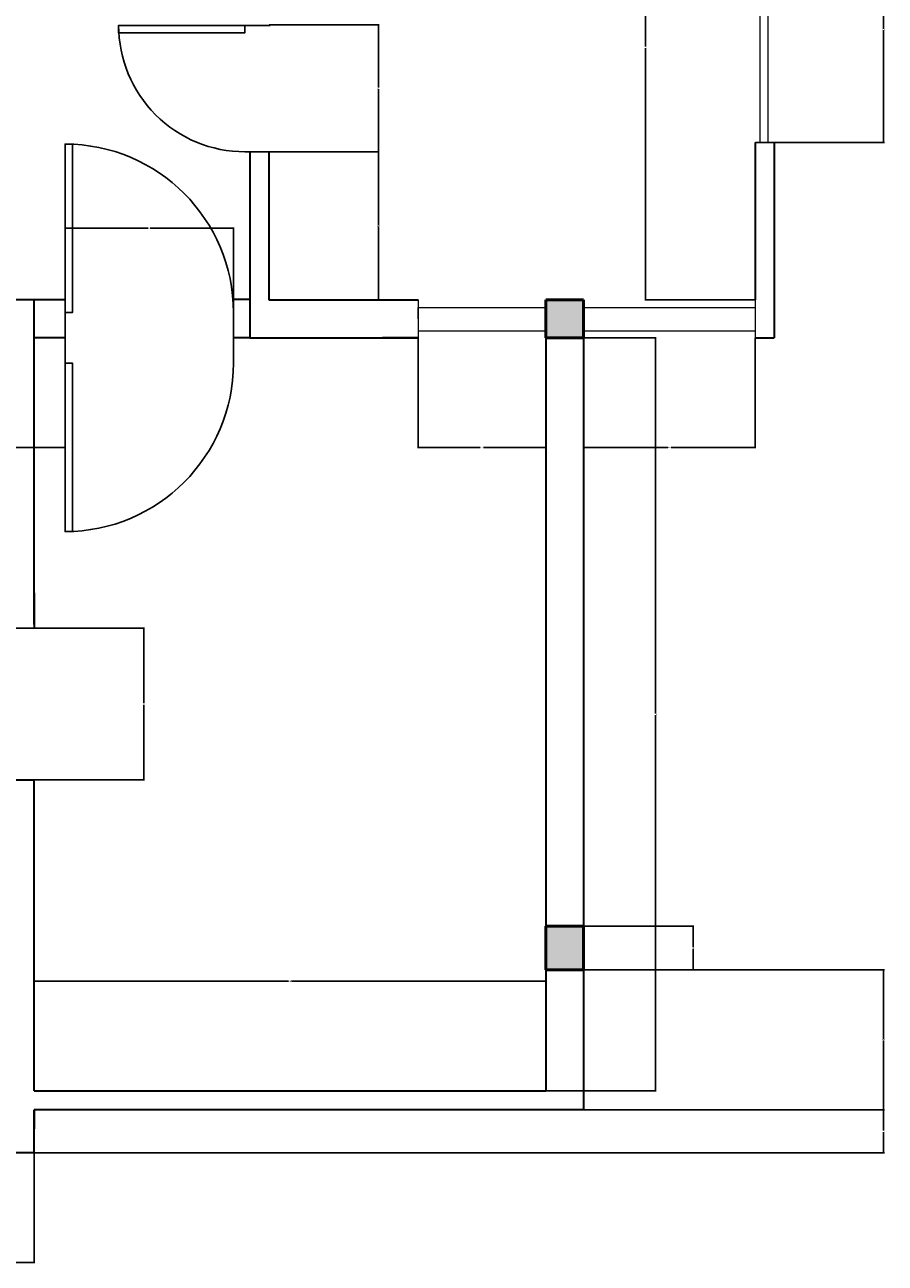
# Model space of a CAD drawing. Units: inches. Extents: x 229 to 651, y 108 to 681.
# Tile 2 of 4: x 447 to 651, y 108 to 402. Entities that reach past the tile are written whole.
import ezdxf

# ---------------------------------------------------------------- set-up
doc = ezdxf.new("R2010")
doc.units = ezdxf.units.IN
doc.header["$MEASUREMENT"] = 0
for name, color, linetype, lineweight in [('A-ANNO-DIMS', 2, 'Continuous', 18), ('A-COLS', 7, 'Continuous', 50), ('A-COLS-PATT', 5, 'Continuous', 13), ('A-DOOR', 3, 'Continuous', 25), ('A-GLAZ', 4, 'Continuous', 18), ('A-WALL', 7, 'Continuous', 35)]:
    doc.layers.add(name, color=color, linetype=linetype, lineweight=lineweight)
doc.styles.get("Standard").update_dxf_attribs({"font": 'arial.ttf'})
doc.dimstyles.get("Standard").update_dxf_attribs({"dimtxt": 0.18, "dimasz": 0.18, "dimexe": 0.18, "dimexo": 0.0625, "dimgap": 0.09, "dimtad": 0, "dimtih": 1, "dimtoh": 1, "dimdec": 4, "dimzin": 0, "dimdsep": 46, "dimtxsty": 'Standard', "dimcen": 0.09, "dimadec": 0, "dimazin": 0, "dimtfac": 1, "dimtdec": 4, "dimtofl": 0, "dimtmove": 0, "dimatfit": 3, "dimfxl": 1, "dimtolj": 1, "dimtzin": 0, "dimarcsym": 0})

# ---------------------------------------------------------------- blocks, each defined once
blk = doc.blocks.new('*U7')
for p, q in [((0, 0), (0, 6)), ((30, 0), (30, 6))]:
    blk.add_line(p, q)
blk.add_lwpolyline([(0, 0), (0, -30), (1.75, -30), (1.75, 0)], close=True)
blk.add_arc((0, 0), 30, 270, 0)
blk = doc.blocks.new('*U2')
for p, q in [((0, 0), (0, -6)), ((40, 0), (40, -6))]:
    blk.add_line(p, q)
blk.add_lwpolyline([(0, 0), (0, 40), (1.75, 40), (1.75, 0)], close=True)
blk.add_arc((0, 0), 40, 0, 90)
blk = doc.blocks.new('*U4')
for p, q in [((0, 0), (0, -6)), ((36, 0), (36, -6))]:
    blk.add_line(p, q)
blk.add_lwpolyline([(0, 0), (0, 36), (1.75, 36), (1.75, 0)], close=True)
blk.add_arc((0, 0), 36, 0, 90)
blk = doc.blocks.new('*D17')
at = {"layer": 'A-ANNO-DIMS', "color": 0, "lineweight": -2, "transparency": 16777216}
for p, q in [((620.41, 457.09), (594.26, 457.09)), ((594.44, 456.91), (594.44, 397.27)), ((594.44, 337.27), (594.44, 396.9)), ((620.41, 337.09), (594.26, 337.09))]:
    blk.add_line(p, q, dxfattribs=at)
at = {"layer": 'A-ANNO-DIMS', "color": 0, "transparency": 16777216}
for points in [[(594.41, 456.91), (594.47, 456.91), (594.44, 457.09)], [(594.41, 337.27), (594.47, 337.27), (594.44, 337.09)]]:
    blk.add_solid(points, dxfattribs=at)
at = {"layer": 'Defpoints', "color": 0, "transparency": 16777216}
for p in [(594.44, 457.09), (620.47, 457.09), (620.47, 337.09)]:
    blk.add_point(p, dxfattribs=at)
at = {"layer": 'A-ANNO-DIMS', "color": 0, "transparency": 16777216, "insert": (594.44, 397.09), "char_height": 0.18, "attachment_point": 5}
blk.add_mtext('\\A1;120', dxfattribs=at)
blk = doc.blocks.new('*D43')
at = {"layer": 'A-ANNO-DIMS', "color": 0, "lineweight": -2, "transparency": 16777216}
for p, q in [((505.03, 402.42), (531.18, 402.42)), ((531, 402.24), (531, 387.52)), ((531, 372.44), (531, 387.15)), ((505.03, 372.26), (531.18, 372.26))]:
    blk.add_line(p, q, dxfattribs=at)
at = {"layer": 'A-ANNO-DIMS', "color": 0, "transparency": 16777216}
for points in [[(530.97, 402.24), (531.03, 402.24), (531, 402.42)], [(530.97, 372.44), (531.03, 372.44), (531, 372.26)]]:
    blk.add_solid(points, dxfattribs=at)
at = {"layer": 'Defpoints', "color": 0, "transparency": 16777216}
for p in [(504.97, 402.42), (504.97, 372.26), (531, 372.26)]:
    blk.add_point(p, dxfattribs=at)
at = {"layer": 'A-ANNO-DIMS', "color": 0, "transparency": 16777216, "insert": (531, 387.34), "char_height": 0.18, "attachment_point": 5}
blk.add_mtext('\\A1;30.16', dxfattribs=at)
blk = doc.blocks.new('*D44')
at = {"layer": 'A-ANNO-DIMS', "color": 0, "lineweight": -2, "transparency": 16777216}
for p, q in [((505.03, 372.26), (531.18, 372.26)), ((531, 372.08), (531, 354.85)), ((531, 337.27), (531, 354.49)), ((505.03, 337.09), (531.18, 337.09))]:
    blk.add_line(p, q, dxfattribs=at)
at = {"layer": 'A-ANNO-DIMS', "color": 0, "transparency": 16777216}
for points in [[(530.97, 372.08), (531.03, 372.08), (531, 372.26)], [(530.97, 337.27), (531.03, 337.27), (531, 337.09)]]:
    blk.add_solid(points, dxfattribs=at)
at = {"layer": 'Defpoints', "color": 0, "transparency": 16777216}
for p in [(504.97, 372.26), (504.97, 337.09), (531, 337.09)]:
    blk.add_point(p, dxfattribs=at)
at = {"layer": 'A-ANNO-DIMS', "color": 0, "transparency": 16777216, "insert": (531, 354.67), "char_height": 0.18, "attachment_point": 5}
blk.add_mtext('\\A1;35.17', dxfattribs=at)
blk = doc.blocks.new('*D45')
at = {"layer": 'A-ANNO-DIMS', "color": 0, "lineweight": -2, "transparency": 16777216}
for p, q in [((620.53, 428.12), (651.18, 428.12)), ((651, 427.94), (651, 401.49)), ((651, 374.68), (651, 401.13)), ((620.53, 374.5), (651.18, 374.5))]:
    blk.add_line(p, q, dxfattribs=at)
at = {"layer": 'A-ANNO-DIMS', "color": 0, "transparency": 16777216}
for points in [[(650.97, 427.94), (651.03, 427.94), (651, 428.12)], [(650.97, 374.68), (651.03, 374.68), (651, 374.5)]]:
    blk.add_solid(points, dxfattribs=at)
at = {"layer": 'Defpoints', "color": 0, "transparency": 16777216}
for p in [(620.47, 428.12), (651, 428.12), (620.47, 374.5)]:
    blk.add_point(p, dxfattribs=at)
at = {"layer": 'A-ANNO-DIMS', "color": 0, "transparency": 16777216, "insert": (651, 401.31), "char_height": 0.18, "attachment_point": 5}
blk.add_mtext('\\A1;53.63', dxfattribs=at)
blk = doc.blocks.new('*D47')
at = {"layer": 'A-ANNO-DIMS', "color": 0, "lineweight": -2, "transparency": 16777216}
for p, q in [((540.4, 328.02), (540.4, 301.88)), ((570.74, 328.02), (570.74, 301.88)), ((540.58, 302.06), (555.18, 302.06)), ((570.56, 302.06), (555.97, 302.06))]:
    blk.add_line(p, q, dxfattribs=at)
at = {"layer": 'A-ANNO-DIMS', "color": 0, "transparency": 16777216}
for points in [[(540.58, 302.09), (540.58, 302.03), (540.4, 302.06)], [(570.56, 302.09), (570.56, 302.03), (570.74, 302.06)]]:
    blk.add_solid(points, dxfattribs=at)
at = {"layer": 'Defpoints', "color": 0, "transparency": 16777216}
for p in [(540.4, 328.09), (570.74, 328.09), (540.4, 302.06)]:
    blk.add_point(p, dxfattribs=at)
at = {"layer": 'A-ANNO-DIMS', "color": 0, "transparency": 16777216, "insert": (555.57, 302.06), "char_height": 0.18, "attachment_point": 5}
blk.add_mtext('\\A1;30.34', dxfattribs=at)
blk = doc.blocks.new('*D48')
at = {"layer": 'A-ANNO-DIMS', "color": 0, "lineweight": -2, "transparency": 16777216}
for p, q in [((579.74, 328.02), (579.74, 301.88)), ((620.47, 328.02), (620.47, 301.88)), ((579.92, 302.06), (599.71, 302.06)), ((620.29, 302.06), (600.5, 302.06))]:
    blk.add_line(p, q, dxfattribs=at)
at = {"layer": 'A-ANNO-DIMS', "color": 0, "transparency": 16777216}
for points in [[(579.92, 302.09), (579.92, 302.03), (579.74, 302.06)], [(620.29, 302.09), (620.29, 302.03), (620.47, 302.06)]]:
    blk.add_solid(points, dxfattribs=at)
at = {"layer": 'Defpoints', "color": 0, "transparency": 16777216}
for p in [(579.74, 328.09), (620.47, 328.09), (579.74, 302.06)]:
    blk.add_point(p, dxfattribs=at)
at = {"layer": 'A-ANNO-DIMS', "color": 0, "transparency": 16777216, "insert": (600.11, 302.06), "char_height": 0.18, "attachment_point": 5}
blk.add_mtext('\\A1;40.73', dxfattribs=at)
blk = doc.blocks.new('*D53')
at = {"layer": 'A-ANNO-DIMS', "color": 0, "lineweight": -2, "transparency": 16777216}
for p, q in [((425.43, 328.02), (425.43, 301.88)), ((456.56, 328.02), (456.56, 301.88)), ((425.61, 302.06), (440.6, 302.06)), ((456.38, 302.06), (441.38, 302.06))]:
    blk.add_line(p, q, dxfattribs=at)
at = {"layer": 'A-ANNO-DIMS', "color": 0, "transparency": 16777216}
for points in [[(425.61, 302.09), (425.61, 302.03), (425.43, 302.06)], [(456.38, 302.09), (456.38, 302.03), (456.56, 302.06)]]:
    blk.add_solid(points, dxfattribs=at)
at = {"layer": 'Defpoints', "color": 0, "transparency": 16777216}
for p in [(425.43, 328.09), (456.56, 328.09), (425.43, 302.06)]:
    blk.add_point(p, dxfattribs=at)
at = {"layer": 'A-ANNO-DIMS', "color": 0, "transparency": 16777216, "insert": (440.99, 302.06), "char_height": 0.18, "attachment_point": 5}
blk.add_mtext('\\A1;31.13', dxfattribs=at)
blk = doc.blocks.new('*D54')
at = {"layer": 'A-ANNO-DIMS', "color": 0, "lineweight": -2, "transparency": 16777216}
for p, q in [((456.56, 328.15), (456.56, 354.3)), ((456.74, 354.12), (476.33, 354.12)), ((496.38, 354.12), (476.78, 354.12)), ((496.56, 328.15), (496.56, 354.3))]:
    blk.add_line(p, q, dxfattribs=at)
at = {"layer": 'A-ANNO-DIMS', "color": 0, "transparency": 16777216}
for points in [[(456.74, 354.15), (456.74, 354.09), (456.56, 354.12)], [(496.38, 354.15), (496.38, 354.09), (496.56, 354.12)]]:
    blk.add_solid(points, dxfattribs=at)
at = {"layer": 'Defpoints', "color": 0, "transparency": 16777216}
for p in [(496.56, 354.12), (456.56, 328.09), (496.56, 328.09)]:
    blk.add_point(p, dxfattribs=at)
at = {"layer": 'A-ANNO-DIMS', "color": 0, "transparency": 16777216, "insert": (476.56, 354.12), "char_height": 0.18, "attachment_point": 5}
blk.add_mtext('\\A1;40', dxfattribs=at)
blk = doc.blocks.new('*D55')
at = {"layer": 'A-ANNO-DIMS', "color": 0, "lineweight": -2, "transparency": 16777216}
for p, q in [((449.24, 149.37), (449.24, 175.52)), ((449.42, 175.34), (509.61, 175.34)), ((570.56, 175.34), (510.38, 175.34)), ((570.74, 149.37), (570.74, 175.52))]:
    blk.add_line(p, q, dxfattribs=at)
at = {"layer": 'A-ANNO-DIMS', "color": 0, "transparency": 16777216}
for points in [[(449.42, 175.37), (449.42, 175.31), (449.24, 175.34)], [(570.56, 175.37), (570.56, 175.31), (570.74, 175.34)]]:
    blk.add_solid(points, dxfattribs=at)
at = {"layer": 'Defpoints', "color": 0, "transparency": 16777216}
for p in [(570.74, 175.34), (449.24, 149.31), (570.74, 149.31)]:
    blk.add_point(p, dxfattribs=at)
at = {"layer": 'A-ANNO-DIMS', "color": 0, "transparency": 16777216, "insert": (509.99, 175.34), "char_height": 0.18, "attachment_point": 5}
blk.add_mtext('\\A1;121.5', dxfattribs=at)
blk = doc.blocks.new('*D56')
at = {"layer": 'A-ANNO-DIMS', "color": 0, "lineweight": -2, "transparency": 16777216}
for p, q in [((579.81, 144.81), (651.18, 144.81)), ((651, 144.63), (651, 139.88)), ((651, 134.77), (651, 139.51)), ((449.31, 134.59), (651.18, 134.59))]:
    blk.add_line(p, q, dxfattribs=at)
at = {"layer": 'A-ANNO-DIMS', "color": 0, "transparency": 16777216}
for points in [[(650.97, 144.63), (651.03, 144.63), (651, 144.81)], [(650.97, 134.77), (651.03, 134.77), (651, 134.59)]]:
    blk.add_solid(points, dxfattribs=at)
at = {"layer": 'Defpoints', "color": 0, "transparency": 16777216}
for p in [(579.74, 144.81), (449.24, 134.59), (651, 134.59)]:
    blk.add_point(p, dxfattribs=at)
at = {"layer": 'A-ANNO-DIMS', "color": 0, "transparency": 16777216, "insert": (651, 139.7), "char_height": 0.18, "attachment_point": 5}
blk.add_mtext('\\A1;10.22', dxfattribs=at)
blk = doc.blocks.new('*D57')
at = {"layer": 'A-ANNO-DIMS', "color": 0, "lineweight": -2, "transparency": 16777216}
for p, q in [((255.74, 134.52), (255.74, 108.38)), ((449.24, 134.52), (449.24, 108.38)), ((255.92, 108.56), (352.11, 108.56)), ((449.06, 108.56), (352.88, 108.56))]:
    blk.add_line(p, q, dxfattribs=at)
at = {"layer": 'A-ANNO-DIMS', "color": 0, "transparency": 16777216}
for points in [[(255.92, 108.59), (255.92, 108.53), (255.74, 108.56)], [(449.06, 108.59), (449.06, 108.53), (449.24, 108.56)]]:
    blk.add_solid(points, dxfattribs=at)
at = {"layer": 'Defpoints', "color": 0, "transparency": 16777216}
for p in [(255.74, 134.59), (449.24, 134.59), (449.24, 108.56)]:
    blk.add_point(p, dxfattribs=at)
at = {"layer": 'A-ANNO-DIMS', "color": 0, "transparency": 16777216, "insert": (352.49, 108.56), "char_height": 0.18, "attachment_point": 5}
blk.add_mtext('\\A1;193.5', dxfattribs=at)
blk = doc.blocks.new('*D58')
at = {"layer": 'A-ANNO-DIMS', "color": 0, "lineweight": -2, "transparency": 16777216}
for p, q in [((570.81, 328.09), (596.95, 328.09)), ((596.77, 327.91), (596.77, 238.88)), ((596.77, 149.49), (596.77, 238.51)), ((570.81, 149.31), (596.95, 149.31))]:
    blk.add_line(p, q, dxfattribs=at)
at = {"layer": 'A-ANNO-DIMS', "color": 0, "transparency": 16777216}
for points in [[(596.74, 327.91), (596.8, 327.91), (596.77, 328.09)], [(596.74, 149.49), (596.8, 149.49), (596.77, 149.31)]]:
    blk.add_solid(points, dxfattribs=at)
at = {"layer": 'Defpoints', "color": 0, "transparency": 16777216}
for p in [(570.74, 328.09), (570.74, 149.31), (596.77, 149.31)]:
    blk.add_point(p, dxfattribs=at)
at = {"layer": 'A-ANNO-DIMS', "color": 0, "transparency": 16777216, "insert": (596.77, 238.7), "char_height": 0.18, "attachment_point": 5}
blk.add_mtext('\\A1;178.78', dxfattribs=at)
blk = doc.blocks.new('*D59')
at = {"layer": 'A-ANNO-DIMS', "color": 0, "lineweight": -2, "transparency": 16777216}
for p, q in [((449.31, 259.15), (475.45, 259.15)), ((475.27, 258.97), (475.27, 241.34)), ((475.27, 223.33), (475.27, 240.97)), ((449.31, 223.15), (475.45, 223.15))]:
    blk.add_line(p, q, dxfattribs=at)
at = {"layer": 'A-ANNO-DIMS', "color": 0, "transparency": 16777216}
for points in [[(475.24, 258.97), (475.3, 258.97), (475.27, 259.15)], [(475.24, 223.33), (475.3, 223.33), (475.27, 223.15)]]:
    blk.add_solid(points, dxfattribs=at)
at = {"layer": 'Defpoints', "color": 0, "transparency": 16777216}
for p in [(449.24, 259.15), (449.24, 223.15), (475.27, 223.15)]:
    blk.add_point(p, dxfattribs=at)
at = {"layer": 'A-ANNO-DIMS', "color": 0, "transparency": 16777216, "insert": (475.27, 241.15), "char_height": 0.18, "attachment_point": 5}
blk.add_mtext('\\A1;36', dxfattribs=at)
blk = doc.blocks.new('*D70')
at = {"layer": 'A-ANNO-DIMS', "color": 0, "lineweight": -2, "transparency": 16777216}
for p, q in [((579.81, 188.43), (605.95, 188.43)), ((605.77, 188.25), (605.77, 183.42)), ((605.77, 178.23), (605.77, 183.06)), ((579.81, 178.05), (605.95, 178.05))]:
    blk.add_line(p, q, dxfattribs=at)
at = {"layer": 'A-ANNO-DIMS', "color": 0, "transparency": 16777216}
for points in [[(605.74, 188.25), (605.8, 188.25), (605.77, 188.43)], [(605.74, 178.23), (605.8, 178.23), (605.77, 178.05)]]:
    blk.add_solid(points, dxfattribs=at)
at = {"layer": 'Defpoints', "color": 0, "transparency": 16777216}
for p in [(579.74, 188.43), (579.74, 178.05), (605.77, 178.05)]:
    blk.add_point(p, dxfattribs=at)
at = {"layer": 'A-ANNO-DIMS', "color": 0, "transparency": 16777216, "insert": (605.77, 183.24), "char_height": 0.18, "attachment_point": 5}
blk.add_mtext('\\A1;10.375', dxfattribs=at)
blk = doc.blocks.new('*D71')
at = {"layer": 'A-ANNO-DIMS', "color": 0, "lineweight": -2, "transparency": 16777216}
for p, q in [((579.81, 178.05), (651.18, 178.05)), ((651, 177.87), (651, 161.61)), ((651, 144.99), (651, 161.25)), ((579.81, 144.81), (651.18, 144.81))]:
    blk.add_line(p, q, dxfattribs=at)
at = {"layer": 'A-ANNO-DIMS', "color": 0, "transparency": 16777216}
for points in [[(650.97, 177.87), (651.03, 177.87), (651, 178.05)], [(650.97, 144.99), (651.03, 144.99), (651, 144.81)]]:
    blk.add_solid(points, dxfattribs=at)
at = {"layer": 'Defpoints', "color": 0, "transparency": 16777216}
for p in [(579.74, 178.05), (651, 178.05), (579.74, 144.81)]:
    blk.add_point(p, dxfattribs=at)
at = {"layer": 'A-ANNO-DIMS', "color": 0, "transparency": 16777216, "insert": (651, 161.43), "char_height": 0.18, "attachment_point": 5}
blk.add_mtext('\\A1;33.244', dxfattribs=at)

msp = doc.modelspace()

# ---------------------------------------------------------------- hatches: boundary and pattern name
at = {"layer": 'A-COLS-PATT'}
h = msp.add_hatch(color=256, dxfattribs=at)
h.dxf.hatch_style = 1
h.paths.add_polyline_path([(264.7698, 655.0869), (255.744, 655.0869), (255.744, 646.0869), (264.7698, 646.0869)])
h.paths.add_polyline_path([(428.5355, 655.0869), (414.8518, 655.0869), (414.8518, 646.0869), (428.5355, 646.0869)])
h.paths.add_polyline_path([(579.744, 655.0869), (568.5366, 655.0869), (568.5366, 646.0869), (570.744, 646.0869), (579.744, 646.0869)])
h.paths.add_polyline_path([(579.744, 468.8158), (570.744, 468.8158), (570.744, 457.0869), (579.744, 457.0869)])
h.paths.add_polyline_path([(422.244, 467.874), (416.0718, 467.874), (416.0718, 457.0869), (422.244, 457.0869)])
h.paths.add_polyline_path([(264.744, 465.8018), (255.744, 465.8018), (255.744, 453.3882), (264.744, 453.3882), (264.744, 457.0869)])
h.paths.add_polyline_path([(264.744, 337.0869), (255.744, 337.0869), (255.744, 328.0161), (264.744, 328.0161)])
h.paths.add_polyline_path([(425.426, 337.0869), (411.84, 337.0869), (411.84, 328.0869), (425.426, 328.0869)])
h.paths.add_polyline_path([(579.744, 337.0869), (570.744, 337.0869), (570.744, 328.0869), (579.744, 328.0869)])
h.paths.add_polyline_path([(579.744, 188.4262), (570.744, 188.4262), (570.744, 178.0508), (579.744, 178.0508)])
h.paths.add_polyline_path([(413.7248, 169.0053), (405.843, 169.0053), (405.843, 162.8404), (413.7248, 162.8404)])
h.paths.add_polyline_path([(264.744, 180.6917), (255.744, 180.6917), (255.744, 171.3369), (264.744, 171.3369)])

# ---------------------------------------------------------------- linework, layer by layer
at = {"layer": 'A-COLS'}
for p, q in [((570.744, 337.0869), (579.744, 337.0869)), ((570.744, 328.0869), (570.744, 337.0869)), ((570.744, 337.0869), (579.744, 337.0869)), ((579.744, 337.0869), (579.744, 328.0869)), ((579.744, 328.0869), (570.744, 328.0869)), ((570.744, 328.0869), (579.744, 328.0869)), ((579.744, 328.0869), (570.744, 328.0869)), ((579.744, 188.4262), (570.744, 188.4262)), ((570.744, 188.4262), (570.744, 178.0508)), ((579.744, 178.0508), (579.744, 188.4262)), ((570.744, 178.0508), (579.744, 178.0508))]:
    msp.add_line(p, q, dxfattribs=at)
at = {"layer": 'A-GLAZ'}
for p, q in [((621.6316, 374.4959), (621.6316, 428.1237)), ((623.4874, 428.1237), (623.4874, 374.4959)), ((620.4705, 374.4959), (624.9705, 374.4959)), ((540.4019, 337.0869), (540.4019, 328.0869)), ((540.4019, 332.5869), (540.4019, 335.2502)), ((540.4019, 335.2502), (570.744, 335.2502)), ((579.744, 335.2502), (620.4705, 335.2502)), ((620.4705, 337.0869), (620.4705, 328.0869)), ((620.4705, 335.2502), (620.4705, 329.7054)), ((570.744, 329.7054), (540.4019, 329.7054)), ((620.4705, 329.7054), (579.744, 329.7054))]:
    msp.add_line(p, q, dxfattribs=at)
at = {"layer": 'A-WALL'}
for p, q in [((620.4705, 374.4959), (620.4705, 337.0869)), ((624.9705, 374.4959), (624.9705, 328.0869)), ((500.4705, 372.2554), (500.4705, 328.0869)), ((504.9705, 372.2554), (504.9705, 337.0869)), ((449.244, 337.0869), (391.5105, 337.0869)), ((456.556, 337.1), (449.244, 337.0869)), ((449.244, 328.0869), (449.244, 337.0869)), ((500.4705, 337.1787), (496.4369, 337.1714)), ((504.9705, 337.0869), (540.4019, 337.0869)), ((531.944, 337.0869), (540.4019, 337.0869)), ((449.244, 260.0214), (449.244, 328.0869)), ((456.556, 328.0869), (449.244, 328.0869)), ((500.4705, 328.0869), (496.556, 328.0869)), ((500.4705, 328.0869), (540.4019, 328.0869)), ((540.4019, 328.0869), (531.944, 328.0869)), ((570.744, 328.0869), (570.744, 149.3063)), ((579.744, 328.0869), (579.744, 144.8063)), ((620.4705, 328.0869), (624.9705, 328.0869)), ((449.244, 260.0214), (449.244, 267.5709)), ((449.244, 267.5709), (449.244, 259.1543)), ((444.744, 223.1543), (449.244, 223.1543)), ((449.244, 149.3063), (449.244, 223.1543)), ((449.244, 149.3063), (570.744, 149.3063)), ((449.244, 143.5869), (449.244, 144.8063)), ((449.244, 144.8063), (449.244, 140.3063)), ((570.744, 144.8063), (449.244, 144.8063)), ((449.244, 134.5869), (449.244, 144.8063)), ((579.744, 144.8063), (570.744, 144.8063)), ((449.244, 134.5869), (268.4408, 134.5869))]:
    msp.add_line(p, q, dxfattribs=at)

# ---------------------------------------------------------------- block references
at = {"layer": 'A-DOOR'}
for name, p, rotation in [('*U7', (499.2945, 402.2554), 270), ('*U4', (443.244, 223.1543), 90)]:
    msp.add_blockref(name, p, dxfattribs=dict(at, rotation=rotation))
msp.add_blockref('*U2', (456.556, 334.0869), dxfattribs=at)
at = {"layer": 'A-DOOR', "xscale": -1, "rotation": 180}
msp.add_blockref('*U2', (456.556, 322.0869), dxfattribs=at)

# ---------------------------------------------------------------- dimensions: what is measured, and where the dimension line sits
at = {"layer": 'A-ANNO-DIMS'}
for base, p1, p2, angle, override, picture, middle in [((594.4405, 457.0869), (620.4705, 337.0869), (620.4705, 457.0869), 90, {"dimdec": 0, "dimlfac": 1, "dimrnd": 0, "dimzin": 0, "dimdsep": 46, "dimlunit": 2}, '*D17', (594.4405, 397.0869)), ((651.0005, 428.1237), (620.4705, 374.4959), (620.4705, 428.1237), 90, {"dimdec": 2, "dimlfac": 1, "dimrnd": 0, "dimzin": 0, "dimdsep": 46, "dimlunit": 2}, '*D45', (651.0005, 401.3098)), ((531.0005, 372.2554), (504.9705, 402.4166), (504.9705, 372.2554), 270, {"dimdec": 2, "dimlfac": 1, "dimrnd": 0, "dimzin": 0, "dimdsep": 46, "dimlunit": 2}, '*D43', (531.0005, 387.336)), ((531.0005, 337.0869), (504.9705, 372.2554), (504.9705, 337.0869), 270, {"dimdec": 2, "dimlfac": 1, "dimrnd": 0, "dimzin": 0, "dimdsep": 46, "dimlunit": 2}, '*D44', (531.0005, 354.6711)), ((425.426, 302.0569), (456.556, 328.0869), (425.426, 328.0869), 180, {"dimdec": 2, "dimlfac": 1, "dimrnd": 0, "dimzin": 0, "dimdsep": 46, "dimlunit": 2}, '*D53', (440.991, 302.0569)), ((540.4019, 302.0569), (570.744, 328.0869), (540.4019, 328.0869), 180, {"dimdec": 2, "dimlfac": 1, "dimrnd": 0, "dimzin": 0, "dimdsep": 46, "dimlunit": 2}, '*D47', (555.5729, 302.0569)), ((596.774, 149.3063), (570.744, 328.0869), (570.744, 149.3063), 270, {"dimdec": 2, "dimlfac": 1, "dimrnd": 0, "dimzin": 0, "dimdsep": 46, "dimlunit": 2}, '*D58', (596.774, 238.6966)), ((579.744, 302.0569), (620.4705, 328.0869), (579.744, 328.0869), 180, {"dimdec": 2, "dimlfac": 1, "dimrnd": 0, "dimzin": 0, "dimdsep": 46, "dimlunit": 2}, '*D48', (600.1073, 302.0569)), ((475.274, 223.1543), (449.244, 259.1543), (449.244, 223.1543), 270, {"dimdec": 0, "dimlfac": 1, "dimrnd": 0, "dimzin": 0, "dimdsep": 46, "dimlunit": 2}, '*D59', (475.274, 241.1543)), ((605.774, 178.0508), (579.744, 188.4262), (579.744, 178.0508), 270, {"dimdec": 3, "dimlfac": 1, "dimrnd": 0, "dimzin": 0, "dimdsep": 46, "dimlunit": 2}, '*D70', (605.774, 183.2385)), ((651.000539, 178.050842), (579.744027, 144.806345), (579.744027, 178.050842), 90, {"dimdec": 3, "dimlfac": 1, "dimrnd": 0, "dimzin": 0, "dimdsep": 46, "dimlunit": 2}, '*D71', (651.000539, 161.428593)), ((651.0005, 134.5869), (579.744, 144.8063), (449.244, 134.5869), 90, {"dimdec": 2, "dimlfac": 1, "dimrnd": 0, "dimzin": 0, "dimdsep": 46, "dimlunit": 2}, '*D56', (651.0005, 139.6966))]:
    dim = msp.add_linear_dim(base=base, p1=p1, p2=p2, angle=angle, dimstyle='Standard', override=override, dxfattribs=at)
    dim.commit()
    dim.dimension.update_dxf_attribs({"geometry": picture, "text_midpoint": middle})
for base, p1, p2, override, picture, middle in [((496.556, 354.1169), (456.556, 328.0869), (496.556, 328.0869), {"dimdec": 0, "dimlfac": 1, "dimrnd": 0, "dimzin": 0, "dimdsep": 46, "dimlunit": 2}, '*D54', (476.556, 354.1169)), ((570.744, 175.3363), (449.244, 149.3063), (570.744, 149.3063), {"dimdec": 1, "dimlfac": 1, "dimrnd": 0, "dimzin": 0, "dimdsep": 46, "dimlunit": 2}, '*D55', (509.994, 175.3363)), ((449.244, 108.5569), (255.744, 134.5869), (449.244, 134.5869), {"dimdec": 1, "dimlfac": 1, "dimrnd": 0, "dimzin": 0, "dimdsep": 46, "dimlunit": 2}, '*D57', (352.494, 108.5569))]:
    dim = msp.add_linear_dim(base=base, p1=p1, p2=p2, dimstyle='Standard', override=override, dxfattribs=at)
    dim.commit()
    dim.dimension.update_dxf_attribs({"geometry": picture, "text_midpoint": middle})

doc.saveas('drawing.dxf')
